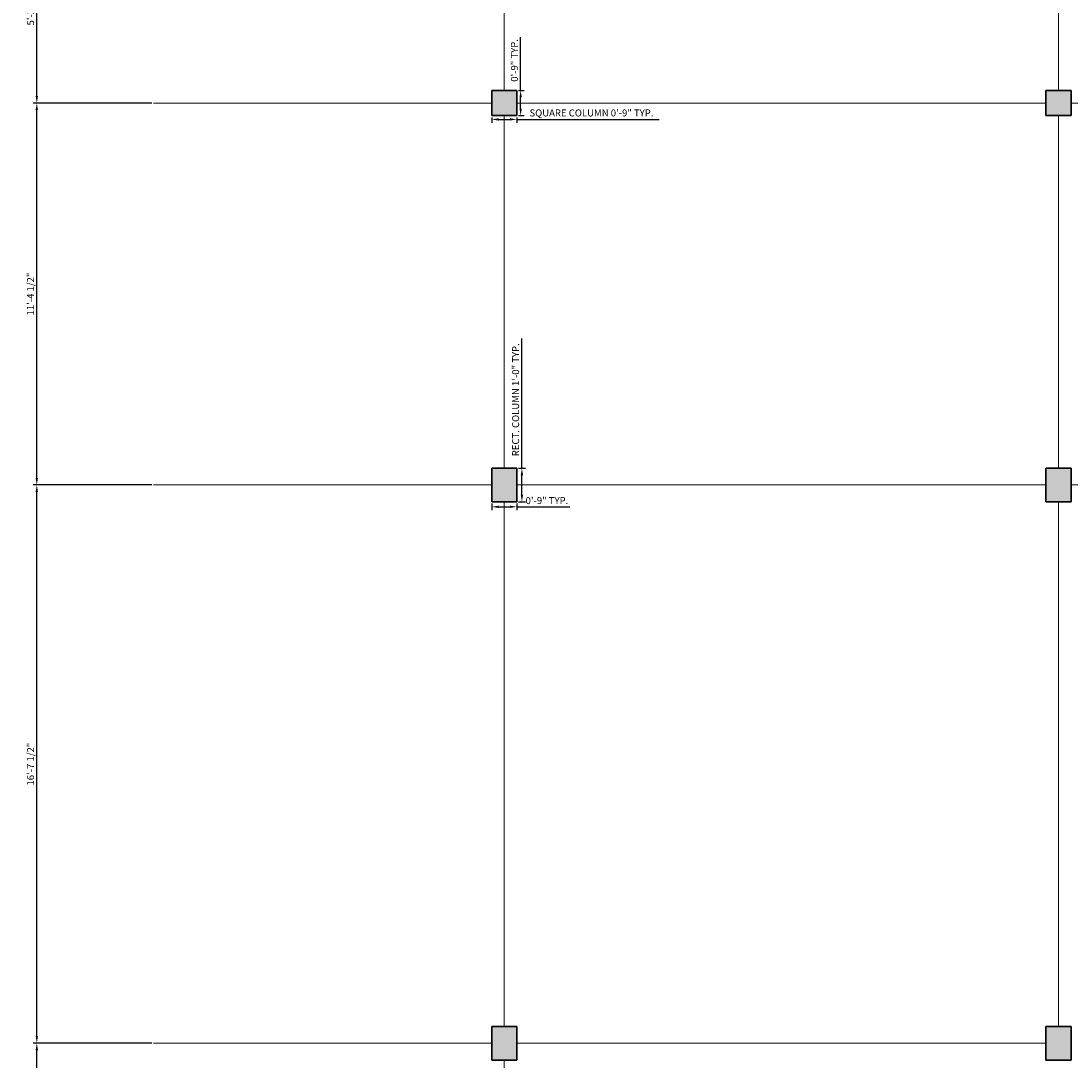
# Model space of a CAD drawing. Units: inches. Extents: x 6038 to 7543, y 3772 to 5131.
# Tile 12 of 14: x 6806 to 7182, y 4547 to 4918. Entities that reach past the tile are written whole.
import ezdxf

# ---------------------------------------------------------------- set-up
doc = ezdxf.new("R2010")
doc.units = ezdxf.units.IN
for name, color, linetype, lineweight in [('A-ANNO-DIMS', 4, 'Continuous', 18), ('S-COLS', 7, 'Continuous', 35), ('S-COLS-PATT', 9, 'Continuous', 13), ('S-GRID', 6, 'Continuous', 13)]:
    doc.layers.add(name, color=color, linetype=linetype, lineweight=lineweight)
doc.styles.get("Standard").update_dxf_attribs({"font": 'arial.ttf'})
doc.dimstyles.new('ISO-25', dxfattribs={"dimtxt": 2.5, "dimasz": 2.5, "dimexe": 1.25, "dimexo": 0.625, "dimtad": 1, "dimdec": 0, "dimlunit": 3, "dimtxsty": 'Standard', "dimcen": 2.5, "dimadec": 0, "dimazin": 0, "dimtfac": 1, "dimtdec": 0, "dimtmove": 0, "dimatfit": 3, "dimfxl": 1, "dimarcsym": 0})

# ---------------------------------------------------------------- blocks, each defined once
blk = doc.blocks.new('COL-9X9')
for p, q in [((0, 9), (9, 9)), ((0, 0), (0, 9)), ((9, 9), (9, 0)), ((9, 0), (0, 0))]:
    blk.add_line(p, q)
blk = doc.blocks.new('COL-9X12')
for p, q in [((0, 12), (9, 12)), ((0, 0), (0, 12)), ((9, 12), (9, 0)), ((9, 0), (0, 0))]:
    blk.add_line(p, q)
blk = doc.blocks.new('*D28')
at = {"layer": 'A-ANNO-DIMS', "color": 0, "lineweight": -2, "transparency": 16777216}
for p, q in [((6974.59, 4883.99), (6974.59, 4882.02)), ((6977.09, 4883.27), (6981.09, 4883.27)), ((6983.59, 4883.99), (6983.59, 4882.02)), ((6983.59, 4883.27), (7034.39, 4883.27))]:
    blk.add_line(p, q, dxfattribs=at)
at = {"layer": 'A-ANNO-DIMS', "color": 0, "transparency": 16777216}
for points in [[(6977.09, 4883.69), (6977.09, 4882.85), (6974.59, 4883.27)], [(6981.09, 4883.69), (6981.09, 4882.85), (6983.59, 4883.27)]]:
    blk.add_solid(points, dxfattribs=at)
at = {"layer": 'Defpoints', "color": 0, "transparency": 16777216}
for p in [(6974.59, 4884.62), (6983.59, 4884.62), (6983.59, 4883.27)]:
    blk.add_point(p, dxfattribs=at)
at = {"layer": 'A-ANNO-DIMS', "color": 0, "transparency": 16777216, "insert": (7010.24, 4885.26), "char_height": 2.5, "attachment_point": 5}
blk.add_mtext('SQUARE COLUMN 0\'-9" TYP.', dxfattribs=at)
blk = doc.blocks.new('*D29')
at = {"layer": 'A-ANNO-DIMS', "color": 0, "lineweight": -2, "transparency": 16777216}
for p, q in [((6984.94, 4893.62), (6984.94, 4912.61)), ((6984.21, 4893.62), (6986.19, 4893.62)), ((6984.94, 4887.12), (6984.94, 4891.12)), ((6984.21, 4884.62), (6986.19, 4884.62))]:
    blk.add_line(p, q, dxfattribs=at)
at = {"layer": 'A-ANNO-DIMS', "color": 0, "transparency": 16777216}
for points in [[(6984.52, 4891.12), (6985.35, 4891.12), (6984.94, 4893.62)], [(6984.52, 4887.12), (6985.35, 4887.12), (6984.94, 4884.62)]]:
    blk.add_solid(points, dxfattribs=at)
at = {"layer": 'Defpoints', "color": 0, "transparency": 16777216}
for p in [(6983.59, 4893.62), (6984.94, 4893.62), (6983.59, 4884.62)]:
    blk.add_point(p, dxfattribs=at)
at = {"layer": 'A-ANNO-DIMS', "color": 0, "transparency": 16777216, "insert": (6983.03, 4904.36), "char_height": 2.5, "attachment_point": 5, "rotation": 90}
blk.add_mtext('0\'-9" TYP.', dxfattribs=at)
blk = doc.blocks.new('*D30')
at = {"layer": 'A-ANNO-DIMS', "color": 0, "lineweight": -2, "transparency": 16777216}
for p, q in [((6985.39, 4758.62), (6985.39, 4805.03)), ((6984.21, 4758.62), (6986.64, 4758.62)), ((6985.39, 4749.12), (6985.39, 4756.12)), ((6984.21, 4746.62), (6986.64, 4746.62))]:
    blk.add_line(p, q, dxfattribs=at)
at = {"layer": 'A-ANNO-DIMS', "color": 0, "transparency": 16777216}
for points in [[(6984.97, 4756.12), (6985.8, 4756.12), (6985.39, 4758.62)], [(6984.97, 4749.12), (6985.8, 4749.12), (6985.39, 4746.62)]]:
    blk.add_solid(points, dxfattribs=at)
at = {"layer": 'Defpoints', "color": 0, "transparency": 16777216}
for p in [(6983.59, 4758.62), (6985.39, 4758.62), (6983.59, 4746.62)]:
    blk.add_point(p, dxfattribs=at)
at = {"layer": 'A-ANNO-DIMS', "color": 0, "transparency": 16777216, "insert": (6983.47, 4783.07), "char_height": 2.5, "attachment_point": 5, "rotation": 90}
blk.add_mtext('RECT. COLUMN 1\'-0" TYP.', dxfattribs=at)
blk = doc.blocks.new('*D31')
at = {"layer": 'A-ANNO-DIMS', "color": 0, "lineweight": -2, "transparency": 16777216}
for p, q in [((6974.59, 4745.99), (6974.59, 4743.57)), ((6977.09, 4744.82), (6981.09, 4744.82)), ((6983.59, 4745.99), (6983.59, 4743.57)), ((6983.59, 4744.82), (7002.57, 4744.82))]:
    blk.add_line(p, q, dxfattribs=at)
at = {"layer": 'A-ANNO-DIMS', "color": 0, "transparency": 16777216}
for points in [[(6977.09, 4745.24), (6977.09, 4744.4), (6974.59, 4744.82)], [(6981.09, 4745.24), (6981.09, 4744.4), (6983.59, 4744.82)]]:
    blk.add_solid(points, dxfattribs=at)
at = {"layer": 'Defpoints', "color": 0, "transparency": 16777216}
for p in [(6974.59, 4746.62), (6983.59, 4746.62), (6983.59, 4744.82)]:
    blk.add_point(p, dxfattribs=at)
at = {"layer": 'A-ANNO-DIMS', "color": 0, "transparency": 16777216, "insert": (6994.33, 4746.72), "char_height": 2.5, "attachment_point": 5}
blk.add_mtext('0\'-9" TYP.', dxfattribs=at)
blk = doc.blocks.new('*D88')
at = {"layer": 'A-ANNO-DIMS', "color": 0, "lineweight": -2, "transparency": 16777216}
for p, q in [((6853.17, 4553.12), (6810.8, 4553.12)), ((6812.05, 4443.12), (6812.05, 4550.62)), ((6853.17, 4440.62), (6810.8, 4440.62))]:
    blk.add_line(p, q, dxfattribs=at)
at = {"layer": 'A-ANNO-DIMS', "color": 0, "transparency": 16777216}
for points in [[(6811.63, 4550.62), (6812.47, 4550.62), (6812.05, 4553.12)], [(6811.63, 4443.12), (6812.47, 4443.12), (6812.05, 4440.62)]]:
    blk.add_solid(points, dxfattribs=at)
at = {"layer": 'Defpoints', "color": 0, "transparency": 16777216}
for p in [(6812.05, 4553.12), (6853.8, 4553.12), (6853.8, 4440.62)]:
    blk.add_point(p, dxfattribs=at)
at = {"layer": 'A-ANNO-DIMS', "color": 0, "transparency": 16777216, "insert": (6810.13, 4496.87), "char_height": 2.5, "attachment_point": 5, "rotation": 90}
blk.add_mtext('9\'-4 1/2"', dxfattribs=at)
blk = doc.blocks.new('*D89')
at = {"layer": 'A-ANNO-DIMS', "color": 0, "lineweight": -2, "transparency": 16777216}
for p, q in [((6853.17, 4752.62), (6810.8, 4752.62)), ((6812.05, 4555.62), (6812.05, 4750.12)), ((6853.17, 4553.12), (6810.8, 4553.12))]:
    blk.add_line(p, q, dxfattribs=at)
at = {"layer": 'A-ANNO-DIMS', "color": 0, "transparency": 16777216}
for points in [[(6811.63, 4750.12), (6812.47, 4750.12), (6812.05, 4752.62)], [(6811.63, 4555.62), (6812.47, 4555.62), (6812.05, 4553.12)]]:
    blk.add_solid(points, dxfattribs=at)
at = {"layer": 'Defpoints', "color": 0, "transparency": 16777216}
for p in [(6812.05, 4752.62), (6853.8, 4752.62), (6853.8, 4553.12)]:
    blk.add_point(p, dxfattribs=at)
at = {"layer": 'A-ANNO-DIMS', "color": 0, "transparency": 16777216, "insert": (6810.13, 4652.87), "char_height": 2.5, "attachment_point": 5, "rotation": 90}
blk.add_mtext('16\'-7 1/2"', dxfattribs=at)
blk = doc.blocks.new('*D90')
at = {"layer": 'A-ANNO-DIMS', "color": 0, "lineweight": -2, "transparency": 16777216}
for p, q in [((6853.17, 4889.12), (6810.8, 4889.12)), ((6812.05, 4755.12), (6812.05, 4886.62)), ((6853.17, 4752.62), (6810.8, 4752.62))]:
    blk.add_line(p, q, dxfattribs=at)
at = {"layer": 'A-ANNO-DIMS', "color": 0, "transparency": 16777216}
for points in [[(6811.63, 4886.62), (6812.47, 4886.62), (6812.05, 4889.12)], [(6811.63, 4755.12), (6812.47, 4755.12), (6812.05, 4752.62)]]:
    blk.add_solid(points, dxfattribs=at)
at = {"layer": 'Defpoints', "color": 0, "transparency": 16777216}
for p in [(6812.05, 4889.12), (6853.8, 4889.12), (6853.8, 4752.62)]:
    blk.add_point(p, dxfattribs=at)
at = {"layer": 'A-ANNO-DIMS', "color": 0, "transparency": 16777216, "insert": (6810.13, 4820.87), "char_height": 2.5, "attachment_point": 5, "rotation": 90}
blk.add_mtext('11\'-4 1/2"', dxfattribs=at)
blk = doc.blocks.new('*D91')
at = {"layer": 'A-ANNO-DIMS', "color": 0, "lineweight": -2, "transparency": 16777216}
for p, q in [((6853.17, 4952.12), (6810.8, 4952.12)), ((6812.05, 4891.62), (6812.05, 4949.62)), ((6853.17, 4889.12), (6810.8, 4889.12))]:
    blk.add_line(p, q, dxfattribs=at)
at = {"layer": 'A-ANNO-DIMS', "color": 0, "transparency": 16777216}
for points in [[(6811.63, 4949.62), (6812.47, 4949.62), (6812.05, 4952.12)], [(6811.63, 4891.62), (6812.47, 4891.62), (6812.05, 4889.12)]]:
    blk.add_solid(points, dxfattribs=at)
at = {"layer": 'Defpoints', "color": 0, "transparency": 16777216}
for p in [(6812.05, 4952.12), (6853.8, 4952.12), (6853.8, 4889.12)]:
    blk.add_point(p, dxfattribs=at)
at = {"layer": 'A-ANNO-DIMS', "color": 0, "transparency": 16777216, "insert": (6810.15, 4920.62), "char_height": 2.5, "attachment_point": 5, "rotation": 90}
blk.add_mtext('5\'-3"', dxfattribs=at)

msp = doc.modelspace()

# ---------------------------------------------------------------- hatches: boundary and pattern name
at = {"layer": 'S-COLS-PATT'}
h = msp.add_hatch(color=256, dxfattribs=at)
h.dxf.hatch_style = 1
h.paths.add_polyline_path([(7325.59, 4944.62), (7334.59, 4944.62), (7334.59, 4956.62), (7325.59, 4956.62)])
h.paths.add_polyline_path([(7334.59, 4746.62), (7334.59, 4758.62), (7325.59, 4758.62), (7325.59, 4746.62)])
h.paths.add_polyline_path([(7181.59, 4758.62), (7172.59, 4758.62), (7172.59, 4746.62), (7181.59, 4746.62)])
h.paths.add_polyline_path([(6983.59, 4758.62), (6974.59, 4758.62), (6974.59, 4746.62), (6983.59, 4746.62)])
h.paths.add_polyline_path([(6983.59, 4559.12), (6974.59, 4559.12), (6974.59, 4547.12), (6983.59, 4547.12)])
h.paths.add_polyline_path([(7181.59, 4559.12), (7172.59, 4559.12), (7172.59, 4547.12), (7181.59, 4547.12)])
h.paths.add_polyline_path([(7334.59, 4559.12), (7325.59, 4559.12), (7325.59, 4547.12), (7334.59, 4547.12)])
h = msp.add_hatch(color=256, dxfattribs=at)
h.dxf.hatch_style = 1
h.paths.add_polyline_path([(6974.59, 4884.62), (6983.59, 4884.62), (6983.59, 4893.62), (6974.59, 4893.62)])
h.paths.add_polyline_path([(7181.59, 4893.62), (7172.59, 4893.62), (7172.59, 4884.62), (7181.59, 4884.62)])
h.paths.add_polyline_path([(6983.59, 4436.12), (6983.59, 4445.12), (6974.59, 4445.12), (6974.59, 4436.12)])
h.paths.add_polyline_path([(7181.59, 4446.62), (7172.59, 4446.62), (7172.59, 4437.62), (7181.59, 4437.62)])
h.paths.add_polyline_path([(7325.59, 4436.12), (7334.59, 4436.12), (7334.59, 4445.12), (7325.59, 4445.12)])
h.paths.add_polyline_path([(7334.59, 4371.62), (7325.59, 4371.62), (7325.59, 4362.62), (7334.59, 4362.62)])
h.paths.add_polyline_path([(7181.59, 4362.62), (7181.59, 4371.62), (7172.59, 4371.62), (7172.59, 4362.62)])
h.paths.add_polyline_path([(6974.59, 4362.62), (6983.59, 4362.62), (6983.59, 4371.62), (6974.59, 4371.62)])

# ---------------------------------------------------------------- linework, layer by layer
at = {"layer": 'S-COLS'}
msp.add_line((6983.59, 4548.62), (6983.59, 4557.62), dxfattribs=at)
at = {"layer": 'S-GRID'}
for p, q in [((6979.09, 5049.84), (6979.09, 4893.62)), ((7177.09, 5049.84), (7177.09, 4893.62)), ((6853.8, 4889.12), (6974.59, 4889.12)), ((6983.59, 4889.12), (7172.59, 4889.12)), ((7181.59, 4889.12), (7450.09, 4889.12)), ((6979.09, 4884.62), (6979.09, 4758.62)), ((7177.09, 4884.62), (7177.09, 4758.62)), ((6974.59, 4752.62), (6853.8, 4752.62)), ((7172.59, 4752.62), (6983.59, 4752.62)), ((7325.59, 4752.62), (7181.59, 4752.62)), ((6979.09, 4746.62), (6979.09, 4559.12)), ((7177.09, 4746.62), (7177.09, 4559.12)), ((6853.8, 4553.12), (6974.59, 4553.12)), ((6983.59, 4553.12), (7172.59, 4553.12)), ((6979.09, 4547.12), (6979.09, 4445.12))]:
    msp.add_line(p, q, dxfattribs=at)

# ---------------------------------------------------------------- block references
at = {"layer": 'S-COLS'}
for name, p in [('COL-9X9', (6974.59, 4884.62)), ('COL-9X9', (7172.59, 4884.62)), ('COL-9X12', (6974.59, 4746.62)), ('COL-9X12', (7172.59, 4746.62)), ('COL-9X12', (6974.59, 4547.12)), ('COL-9X12', (7172.59, 4547.12))]:
    msp.add_blockref(name, p, dxfattribs=at)

# ---------------------------------------------------------------- dimensions: what is measured, and where the dimension line sits
at = {"layer": 'A-ANNO-DIMS'}
for base, p1, p2, picture, middle in [((6812.05, 4952.12), (6853.8, 4889.12), (6853.8, 4952.12), '*D91', (6810.15, 4920.62)), ((6812.05, 4889.12), (6853.8, 4752.62), (6853.8, 4889.12), '*D90', (6810.13, 4820.87)), ((6812.05, 4752.62), (6853.8, 4553.12), (6853.8, 4752.62), '*D89', (6810.13, 4652.87)), ((6812.05, 4553.12), (6853.8, 4440.62), (6853.8, 4553.12), '*D88', (6810.13, 4496.87))]:
    dim = msp.add_linear_dim(base=base, p1=p1, p2=p2, angle=90, dimstyle='ISO-25', override={"dimdec": 1, "dimlfac": 1, "dimrnd": 0, "dimzin": 1, "dimdsep": 46, "dimlunit": 4, "dimfrac": 2}, dxfattribs=at)
    dim.commit()
    dim.dimension.update_dxf_attribs({"geometry": picture, "text_midpoint": middle})
for base, p1, p2, text, picture, middle in [((6984.94, 4893.62), (6983.59, 4884.62), (6983.59, 4893.62), '<> TYP.', '*D29', (6983.03, 4904.36)), ((6985.39, 4758.62), (6983.59, 4746.62), (6983.59, 4758.62), 'RECT. COLUMN <> TYP.', '*D30', (6983.47, 4783.07))]:
    dim = msp.add_linear_dim(base=base, p1=p1, p2=p2, angle=90, text=text, dimstyle='ISO-25', override={"dimdec": 1, "dimlfac": 1, "dimrnd": 0, "dimzin": 1, "dimdsep": 46, "dimlunit": 4, "dimfrac": 2}, dxfattribs=at)
    dim.commit()
    dim.dimension.update_dxf_attribs({"geometry": picture, "text_midpoint": middle})
for base, p1, p2, text, picture, middle in [((6983.59, 4883.27), (6974.59, 4884.62), (6983.59, 4884.62), 'SQUARE COLUMN <> TYP.', '*D28', (7010.24, 4885.26)), ((6983.59, 4744.82), (6974.59, 4746.62), (6983.59, 4746.62), '<> TYP.', '*D31', (6994.33, 4746.72))]:
    dim = msp.add_linear_dim(base=base, p1=p1, p2=p2, text=text, dimstyle='ISO-25', override={"dimdec": 1, "dimlfac": 1, "dimrnd": 0, "dimzin": 1, "dimdsep": 46, "dimlunit": 4, "dimfrac": 2}, dxfattribs=at)
    dim.commit()
    dim.dimension.update_dxf_attribs({"geometry": picture, "text_midpoint": middle})

doc.saveas('drawing.dxf')
